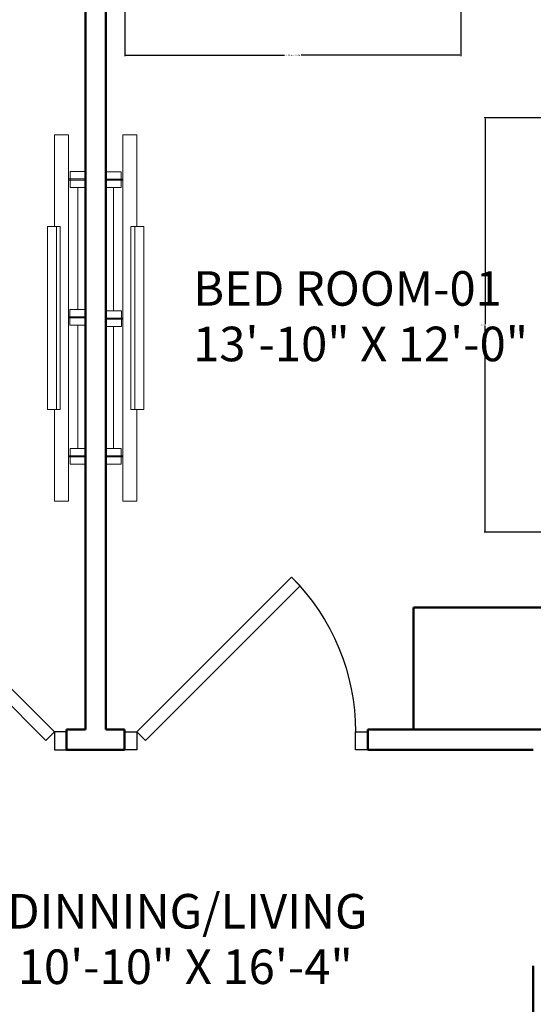
# Model space of a CAD drawing. Units: inches. Extents: x 64 to 1167, y 117 to 939.
# Tile 19 of 56: x 284 to 385, y 583 to 777. Entities that reach past the tile are written whole.
import ezdxf

# ---------------------------------------------------------------- set-up
doc = ezdxf.new("R2010")
doc.units = ezdxf.units.IN
doc.header["$MEASUREMENT"] = 0
for name, color, linetype, lineweight in [('A-ANNO-DIMS', 2, 'Continuous', 18), ('A-ANNO-TEXT', 7, 'Continuous', 25), ('A-DOOR', 4, 'Continuous', 25), ('A-FLOR-FIXT', 8, 'Continuous', 18), ('A-WALL', 7, 'Continuous', 50)]:
    doc.layers.add(name, color=color, linetype=linetype, lineweight=lineweight)
doc.styles.get("Standard").update_dxf_attribs({"font": 'arial.ttf'})
doc.dimstyles.get("Standard").update_dxf_attribs({"dimtxt": 0.18, "dimasz": 0.18, "dimexe": 0.18, "dimexo": 0.0625, "dimgap": 0.09, "dimtad": 0, "dimtih": 1, "dimtoh": 1, "dimdec": 4, "dimzin": 0, "dimdsep": 46, "dimtxsty": 'Standard', "dimcen": 0.09, "dimadec": 0, "dimazin": 0, "dimtfac": 1, "dimtdec": 4, "dimtofl": 0, "dimtmove": 0, "dimatfit": 3, "dimfxl": 1, "dimtolj": 1, "dimtzin": 0, "dimarcsym": 0})

# ---------------------------------------------------------------- blocks, each defined once
blk = doc.blocks.new('A$C68901CC0')
for p, q in [((10.95466834153159, 26.61577842384394), (12.3466108238266, 28.00772090643226)), ((12.3466108238266, 28.00772090643226), (37.40157551217649, 2.952756218669026)), ((36.00963302988149, 1.560813736080697), (10.95466834153159, 26.61577842384394)), ((7.090268874e-07, 2.952756218669026), (7.090268874e-07, 3.131572157e-07)), ((1.968504646034761, 2.952756218669026), (7.090268874e-07, 2.952756218669026)), ((1.968504646034761, 3.131572157e-07), (1.968504646034761, 2.952756218669026)), ((37.40157551217649, 2.952756218669026), (36.00963302988149, 1.560813736080697)), ((37.40157551217649, 2.952756218669026), (37.40157551217649, 3.131572157e-07)), ((39.37007944918437, 2.952756218669026), (37.40157551217649, 2.952756218669026)), ((39.37007944918437, 3.131572157e-07), (39.37007944918437, 2.952756218669026)), ((7.090268874e-07, 3.131572157e-07), (1.968504646034761, 3.131572157e-07)), ((37.40157551217649, 3.131572157e-07), (39.37007944918437, 3.131572157e-07))]:
    blk.add_line(p, q)
blk.add_arc((37.40157551371189, 2.952756218643245), 35.43307086614174, 135.0000000005895, 180)
blk = doc.blocks.new("FLAT TV 6'")
for p, q in [((2564.732677128855, 835.7296006426437), (2564.732677128855, 838.9908005795412)), ((2564.972677128855, 835.7296006426437), (2564.972677128855, 838.9908005795412)), ((2591.807340898264, 835.6699006268682), (2591.807340898264, 838.9311005637654)), ((2592.047340898264, 835.6699006268682), (2592.047340898264, 838.9311005637654)), ((2619.134613045678, 835.7296006426437), (2619.134613045678, 838.9908005795412)), ((2619.374613045678, 835.7296006426437), (2619.374613045678, 838.9908005795412)), ((2566.414374096518, 837.4908005795411), (2590.365643930601, 837.4908005795411)), ((2593.489037865927, 837.4908005795411), (2617.692916078015, 837.4908005795411)), ((2556.053645087266, 835.6699006268682), (2628.053645087266, 835.6699006268682)), ((2556.053645087266, 832.9199006268682), (2556.053645087267, 835.6699006268682)), ((2628.053645087266, 832.9199006268682), (2628.053645087266, 835.6699006268682)), ((2556.053645087267, 832.9199006268682), (2574.053645087266, 832.9199006268682)), ((2574.053645087266, 831.5449006268682), (2574.053645087266, 834.0449006268681)), ((2574.053645087266, 834.0449006268681), (2610.053645087266, 834.0449006268681)), ((2574.053645087266, 833.2949006268682), (2610.053645087266, 833.2949006268682)), ((2610.053645087266, 834.0449006268681), (2610.053645087266, 831.5449006268682)), ((2610.053645087266, 832.9199006268682), (2628.053645087266, 832.9199006268682)), ((2574.053645087266, 831.5449006268682), (2610.053645087266, 831.5449006268682))]:
    blk.add_line(p, q)
for points in [[(2563.290980161192, 838.9908005795412), (2566.414374096518, 838.9908005795412), (2566.414374096518, 835.9908005795412), (2563.290980161192, 835.9908005795412)], [(2590.365643930601, 838.9311005637654), (2593.489037865927, 838.9311005637654), (2593.489037865927, 835.9311005637655), (2590.365643930601, 835.9311005637655)], [(2620.816310013341, 838.9908005795412), (2617.692916078015, 838.9908005795412), (2617.692916078015, 835.9908005795412), (2620.816310013341, 835.9908005795412)]]:
    blk.add_lwpolyline(points, close=True)
blk = doc.blocks.new('*D78')
at = {"layer": 'A-ANNO-DIMS', "color": 0, "lineweight": -2, "transparency": 16777216}
for p, q in [((387.7903462954009, 757.4471057688899), (375.4623196080605, 757.4471057688899)), ((375.6423196080604, 757.26710576889), (375.6423196080604, 716.9284811130437)), ((375.6423196080604, 676.2235945199534), (375.6423196080604, 716.5622191757996)), ((387.7903462954009, 676.0435945199534), (375.4623196080605, 676.0435945199534))]:
    blk.add_line(p, q, dxfattribs=at)
for points in [[(375.6123196080605, 757.26710576889), (375.6723196080604, 757.26710576889), (375.6423196080604, 757.4471057688899)], [(375.6123196080605, 676.2235945199534), (375.6723196080604, 676.2235945199534), (375.6423196080604, 676.0435945199534)]]:
    blk.add_solid(points, dxfattribs=at)
at = {"layer": 'Defpoints', "color": 0, "lineweight": -2, "transparency": 16777216}
for p in [(387.8528462954009, 757.4471057688899), (375.6423196080604, 676.0435945199534), (387.8528462954009, 676.0435945199534)]:
    blk.add_point(p, dxfattribs=at)
at = {"layer": 'A-ANNO-DIMS', "color": 0, "transparency": 16777216, "insert": (375.6423196080606, 716.7453501444215), "char_height": 0.18, "attachment_point": 5}
blk.add_mtext('\\A1;DOUBLE BED 81', dxfattribs=at)
blk = doc.blocks.new('*D94')
at = {"layer": 'A-ANNO-DIMS', "color": 0, "lineweight": -2, "transparency": 16777216}
for p, q in [((304.8599537008231, 779.6380906485667), (304.8599537008231, 769.6205906485667)), ((370.8599537008232, 779.6380906485667), (370.8599537008232, 769.6205906485667)), ((305.0399537008231, 769.8005906485668), (336.2371910814507, 769.8005906485668)), ((370.6799537008232, 769.8005906485668), (339.4827163201956, 769.8005906485668))]:
    blk.add_line(p, q, dxfattribs=at)
for points in [[(305.0399537008231, 769.8305906485667), (305.0399537008231, 769.7705906485667), (304.8599537008231, 769.8005906485668)], [(370.6799537008232, 769.8305906485667), (370.6799537008232, 769.7705906485667), (370.8599537008232, 769.8005906485668)]]:
    blk.add_solid(points, dxfattribs=at)
at = {"layer": 'Defpoints', "color": 0, "lineweight": -2, "transparency": 16777216}
for p in [(304.8599537008231, 779.7005906485667), (370.8599537008232, 779.7005906485667), (370.8599537008232, 769.8005906485668)]:
    blk.add_point(p, dxfattribs=at)
at = {"layer": 'A-ANNO-DIMS', "color": 0, "transparency": 16777216, "insert": (337.8599537008232, 769.8005906485668), "char_height": 0.18, "attachment_point": 5}
blk.add_mtext('\\A1;SLIDING GLASS DOOR 66', dxfattribs=at)

msp = doc.modelspace()

# ---------------------------------------------------------------- linework, layer by layer
at = {"layer": 'A-WALL'}
for p, q in [((297.1072888543381, 781.1997537567942), (297.1072888543382, 637.1997537567942)), ((301.1072888543381, 781.1997537567942), (301.1072888543381, 637.1997537567942)), ((467.107288854338, 661.1997537567942), (361.596672602729, 661.1997537567942)), ((361.5966726027291, 661.1997537567942), (361.5966726027291, 637.1997537567942)), ((297.1072888543381, 637.1997537567942), (293.3769966302316, 637.1997537567942)), ((293.3769966302316, 637.1997537567942), (293.3769966302316, 633.1997537567943)), ((304.7957868632612, 637.1997537567942), (301.1072888543381, 637.1997537567942)), ((304.7957868632612, 637.1997537567942), (304.7957868632612, 633.1997537567943)), ((467.107288854338, 637.1997537567942), (352.56373468102, 637.1997537567942)), ((352.56373468102, 637.1997537567942), (352.5637346810201, 633.1997537567943)), ((304.7957868632612, 633.1997537567943), (293.3769966302316, 633.1997537567943)), ((385.107288854338, 633.1997537567943), (352.5637346810201, 633.1997537567943)), ((385.1072888543381, 590.7850430446796), (385.107288854338, 581.1997537567942))]:
    msp.add_line(p, q, dxfattribs=at)

# ---------------------------------------------------------------- block references
at = {"layer": 'A-DOOR', "yscale": 1.213305874571074, "zscale": 1.213305874571074}
for p, xscale in [((245.6090479522063, 633.1997533768388), 1.213305874571074), ((352.5637355412865, 633.1997533768388), -1.213305874571074)]:
    msp.add_blockref('A$C68901CC0', p, dxfattribs=dict(at, xscale=xscale))
at = {"layer": 'A-FLOR-FIXT'}
for p, rotation in [((-541.8835117252027, 3310.189831433517), 270), ((1140.098089433879, -1873.93417625263), 89.99999999999999)]:
    msp.add_blockref("FLAT TV 6'", p, dxfattribs=dict(at, rotation=rotation))

# ---------------------------------------------------------------- texts
at = {"layer": 'A-ANNO-TEXT'}
for s, p in [('BED ROOM-01', (318.2589031039697, 720.537456162564)), ('13\'-10" X 12\'-0"', (318.2589031039697, 709.6255453390143)), ('DINNING/LIVING', (281.7325571441879, 598.0971709452933)), (' 10\'-10" X 16\'-4"', (281.7325571441879, 587.1852601217435))]:
    msp.add_text(s, height=6.792722406506982, dxfattribs=at).set_placement(p)

# ---------------------------------------------------------------- dimensions: what is measured, and where the dimension line sits
at = {"layer": 'A-ANNO-DIMS'}
dim = msp.add_linear_dim(base=(370.8599537008232, 769.8005906485668), p1=(304.8599537008231, 779.7005906485667), p2=(370.8599537008232, 779.7005906485667), text='SLIDING GLASS DOOR <>', dimstyle='Standard', override={"dimdec": 0, "dimlfac": 1, "dimrnd": 0, "dimzin": 0, "dimdsep": 46, "dimlunit": 2}, dxfattribs=at)
dim.commit()
dim.dimension.update_dxf_attribs({"geometry": '*D94', "text_midpoint": (337.8599537008232, 769.8005906485668)})
dim = msp.add_linear_dim(base=(375.6423196080604, 676.0435945199534), p1=(387.8528462954007, 757.4471057688897), p2=(387.8528462954007, 676.0435945199532), angle=270, text='DOUBLE BED <>', dimstyle='Standard', override={"dimdec": 0, "dimlfac": 1, "dimrnd": 0, "dimzin": 0, "dimdsep": 46, "dimlunit": 2}, dxfattribs=at)
dim.commit()
dim.dimension.update_dxf_attribs({"geometry": '*D78', "text_midpoint": (375.6423196080606, 716.7453501444215)})

doc.saveas('drawing.dxf')
